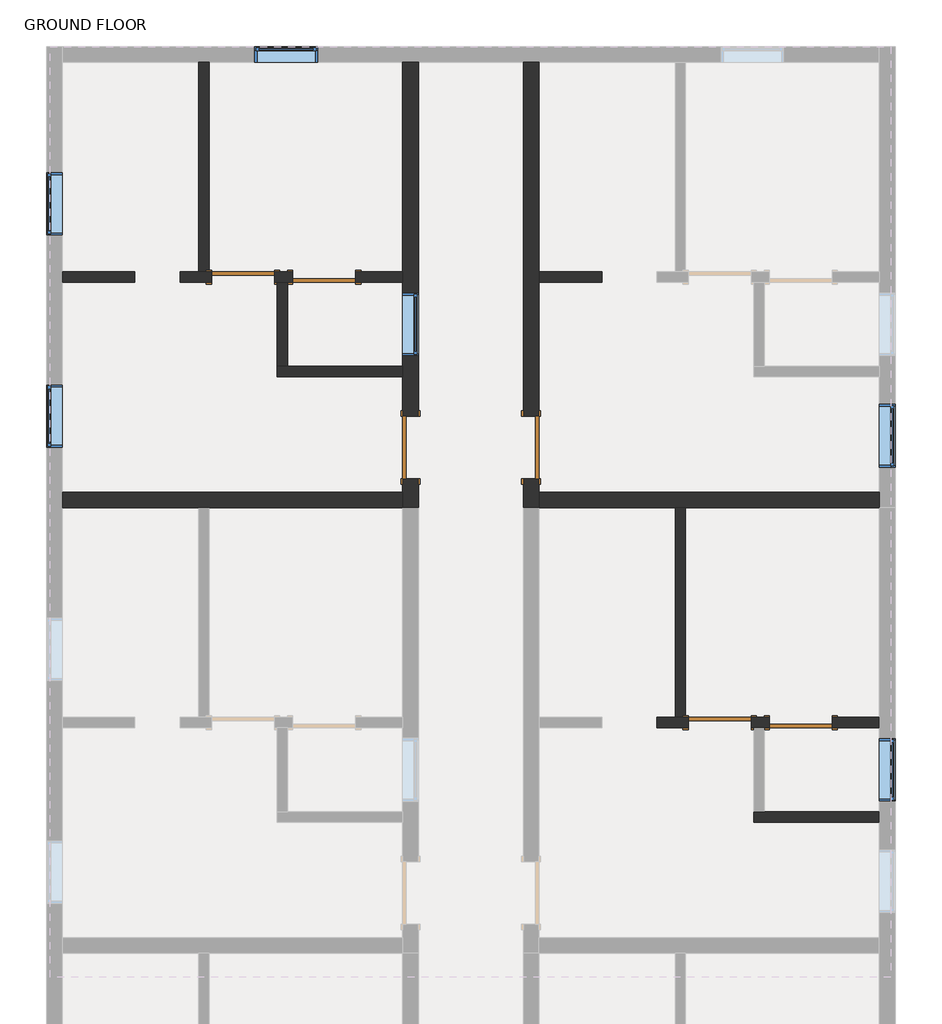
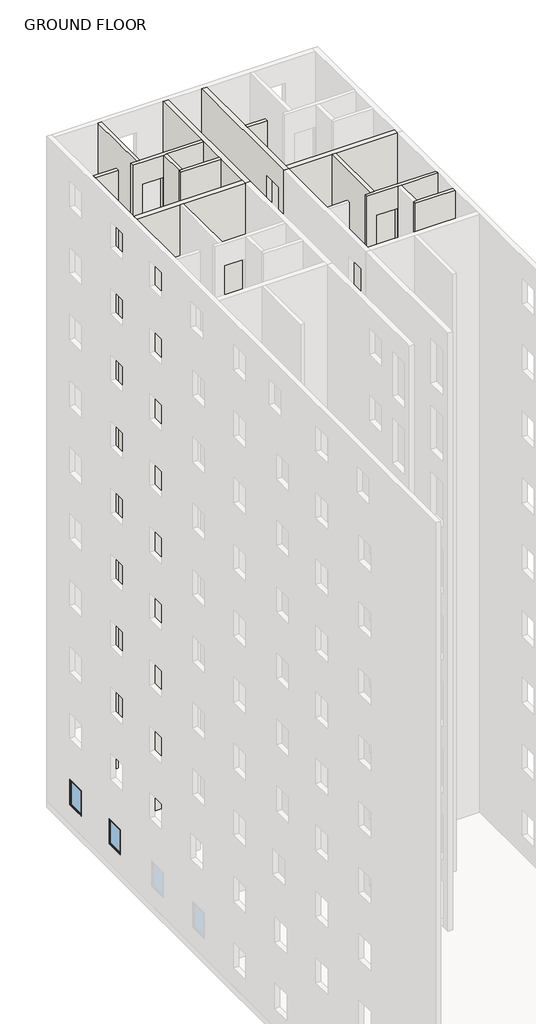
# One storey, part 6 of 7: 13 walls, 6 doors, 6 windows.
"""IFC4 building model written with IfcOpenShell, lengths in millimetres."""

from ifc_helpers import new_model, si_unit, origin, origin_with_axes, place, context, project, spatial, polyline, outline, extrude, faceted_brep, transform, mapped, element, save
from components import door_686f89d2, door_16372e1c, door_a90ba1ad, door_0ca8825f, window_c1f32544

model = new_model("IFC4")

# Units and contexts
model_context = context("Model", 3, world=origin())
ifc_project = project(units=[si_unit("LENGTHUNIT", "METRE", prefix="MILLI")], contexts=[model_context])

# Site, building, storey
site = spatial("IfcSite", under=ifc_project)
building = spatial("IfcBuilding", under=site)
storey = spatial("IfcBuildingStorey", under=building, Name="GROUND FLOOR", Elevation=0.0)

# Doors
placement = place(None, origin())
door_shape = door_686f89d2(model_context)
element("IfcDoor", 1, ObjectType="Single-Flush : 36\" x 84\"", at=placement, inside=storey, context=model_context, shape_type="MappedRepresentation", body=[
    mapped(door_shape, transform((-9863.5902461, 11952.2710592, 0.0), x_axis=(-1.0, 0.0, 0.0), y_axis=(0.0, -1.0, 0.0), z_axis=(0.0, 0.0, 1.0))),
])
element("IfcDoor", 2, ObjectType="Single-Flush : 36\" x 84\"", at=placement, inside=storey, context=model_context, shape_type="MappedRepresentation", body=[
    mapped(door_shape, transform((-2929.3902461, 5475.2710592, 0.0), x_axis=(-1.0, 0.0, 0.0), y_axis=(0.0, -1.0, 0.0), z_axis=(0.0, 0.0, 1.0))),
])
door_2_shape = door_16372e1c(model_context)
element("IfcDoor", 3, ObjectType="Single-Flush : 36\" x 84\"", at=placement, inside=storey, context=model_context, shape_type="MappedRepresentation", body=[
    mapped(door_2_shape, transform((-8682.4902461, 11952.2710592, 0.0), x_axis=(-1.0, 0.0, 0.0), y_axis=(0.0, -1.0, 0.0), z_axis=(0.0, 0.0, 1.0))),
])
element("IfcDoor", 4, ObjectType="Single-Flush : 36\" x 84\"", at=placement, inside=storey, context=model_context, shape_type="MappedRepresentation", body=[
    mapped(door_2_shape, transform((-1748.2902461, 5475.2710592, 0.0), x_axis=(-1.0, 0.0, 0.0), y_axis=(0.0, -1.0, 0.0), z_axis=(0.0, 0.0, 1.0))),
])
door_3_shape = door_a90ba1ad(model_context)
element("IfcDoor", 5, ObjectType="Single-Flush : 36\" x 84\"", at=placement, inside=storey, context=model_context, shape_type="MappedRepresentation", body=[
    mapped(door_3_shape, transform((-7425.1902461, 9475.7710592, 0.0), x_axis=(0.0, -1.0, 0.0), y_axis=(1.0, 0.0, 0.0), z_axis=(0.0, 0.0, 1.0))),
])
door_4_shape = door_0ca8825f(model_context)
element("IfcDoor", 6, ObjectType="Single-Flush : 36\" x 84\"", at=placement, inside=storey, context=model_context, shape_type="MappedRepresentation", body=[
    mapped(door_4_shape, transform((-5672.5902461, 9475.7710592, 0.0), x_axis=(0.0, -1.0, 0.0), y_axis=(1.0, 0.0, 0.0), z_axis=(0.0, 0.0, 1.0))),
])

# Walls
element("IfcWall", 7, ObjectType="Generic - 8\"", at=placement, inside=storey, context=model_context, shape_type="Brep", body=[
    faceted_brep([(-5558.2902461, 8599.4710592, 0.0), (-5558.2902461, 8828.0710592, 0.0), (-5558.2902461, 9018.5710592, 0.0), (-5558.2902461, 9018.5710592, 2133.6), (-5558.2902461, 9932.9710592, 2133.6), (-5558.2902461, 9932.9710592, 0.0), (-5558.2902461, 11876.0710592, 0.0), (-5558.2902461, 12028.4710592, 0.0), (-5558.2902461, 15076.4710592, 0.0), (-5558.2902461, 15076.4710592, 32004.0), (-5558.2902461, 12028.4710592, 32004.0), (-5558.2902461, 11876.0710592, 32004.0), (-5558.2902461, 8828.0710592, 32004.0), (-5558.2902461, 8599.4710592, 32004.0), (-5558.2902461, 9932.9710592, 3200.4), (-5558.2902461, 9018.5710592, 3200.4), (-5558.2902461, 9018.5710592, 5334.0), (-5558.2902461, 9932.9710592, 5334.0), (-5558.2902461, 9932.9710592, 6400.8), (-5558.2902461, 9018.5710592, 6400.8), (-5558.2902461, 9018.5710592, 8534.4), (-5558.2902461, 9932.9710592, 8534.4), (-5558.2902461, 9932.9710592, 9601.2), (-5558.2902461, 9018.5710592, 9601.2), (-5558.2902461, 9018.5710592, 11734.8), (-5558.2902461, 9932.9710592, 11734.8), (-5558.2902461, 9932.9710592, 12801.6), (-5558.2902461, 9018.5710592, 12801.6), (-5558.2902461, 9018.5710592, 14935.2), (-5558.2902461, 9932.9710592, 14935.2), (-5558.2902461, 9932.9710592, 16002.0), (-5558.2902461, 9018.5710592, 16002.0), (-5558.2902461, 9018.5710592, 18135.6), (-5558.2902461, 9932.9710592, 18135.6), (-5558.2902461, 9932.9710592, 19202.4), (-5558.2902461, 9018.5710592, 19202.4), (-5558.2902461, 9018.5710592, 21336.0), (-5558.2902461, 9932.9710592, 21336.0), (-5558.2902461, 9932.9710592, 22402.8), (-5558.2902461, 9018.5710592, 22402.8), (-5558.2902461, 9018.5710592, 24536.4), (-5558.2902461, 9932.9710592, 24536.4), (-5558.2902461, 9932.9710592, 25603.2), (-5558.2902461, 9018.5710592, 25603.2), (-5558.2902461, 9018.5710592, 27736.8), (-5558.2902461, 9932.9710592, 27736.8), (-5558.2902461, 9932.9710592, 28803.6), (-5558.2902461, 9018.5710592, 28803.6), (-5558.2902461, 9018.5710592, 30937.2), (-5558.2902461, 9932.9710592, 30937.2), (-5786.8902461, 9018.5710592, 2133.6), (-5786.8902461, 9018.5710592, 0.0), (-5786.8902461, 8599.4710592, 0.0), (-5786.8902461, 8599.4710592, 32004.0), (-5786.8902461, 15076.4710592, 32004.0), (-5786.8902461, 15076.4710592, 0.0), (-5786.8902461, 9932.9710592, 0.0), (-5786.8902461, 9932.9710592, 2133.6), (-5786.8902461, 9932.9710592, 3200.4), (-5786.8902461, 9932.9710592, 5334.0), (-5786.8902461, 9018.5710592, 5334.0), (-5786.8902461, 9018.5710592, 3200.4), (-5786.8902461, 9932.9710592, 6400.8), (-5786.8902461, 9932.9710592, 8534.4), (-5786.8902461, 9018.5710592, 8534.4), (-5786.8902461, 9018.5710592, 6400.8), (-5786.8902461, 9932.9710592, 9601.2), (-5786.8902461, 9932.9710592, 11734.8), (-5786.8902461, 9018.5710592, 11734.8), (-5786.8902461, 9018.5710592, 9601.2), (-5786.8902461, 9932.9710592, 12801.6), (-5786.8902461, 9932.9710592, 14935.2), (-5786.8902461, 9018.5710592, 14935.2), (-5786.8902461, 9018.5710592, 12801.6), (-5786.8902461, 9932.9710592, 16002.0), (-5786.8902461, 9932.9710592, 18135.6), (-5786.8902461, 9018.5710592, 18135.6), (-5786.8902461, 9018.5710592, 16002.0), (-5786.8902461, 9932.9710592, 19202.4), (-5786.8902461, 9932.9710592, 21336.0), (-5786.8902461, 9018.5710592, 21336.0), (-5786.8902461, 9018.5710592, 19202.4), (-5786.8902461, 9932.9710592, 22402.8), (-5786.8902461, 9932.9710592, 24536.4), (-5786.8902461, 9018.5710592, 24536.4), (-5786.8902461, 9018.5710592, 22402.8), (-5786.8902461, 9932.9710592, 25603.2), (-5786.8902461, 9932.9710592, 27736.8), (-5786.8902461, 9018.5710592, 27736.8), (-5786.8902461, 9018.5710592, 25603.2), (-5786.8902461, 9932.9710592, 28803.6), (-5786.8902461, 9932.9710592, 30937.2), (-5786.8902461, 9018.5710592, 30937.2), (-5786.8902461, 9018.5710592, 28803.6)], [[[0, 1, 2, 3, 4, 5, 6, 7, 8, 9, 10, 11, 12, 13], [14, 15, 16, 17], [18, 19, 20, 21], [22, 23, 24, 25], [26, 27, 28, 29], [30, 31, 32, 33], [34, 35, 36, 37], [38, 39, 40, 41], [42, 43, 44, 45], [46, 47, 48, 49]], [[50, 51, 52, 53, 54, 55, 56, 57], [58, 59, 60, 61], [62, 63, 64, 65], [66, 67, 68, 69], [70, 71, 72, 73], [74, 75, 76, 77], [78, 79, 80, 81], [82, 83, 84, 85], [86, 87, 88, 89], [90, 91, 92, 93]], [[56, 55, 8, 7, 6, 5]], [[52, 51, 2, 1, 0]], [[13, 12, 11, 10, 9, 54, 53]], [[0, 13, 53, 52]], [[9, 8, 55, 54]], [[3, 2, 51, 50]], [[4, 3, 50, 57]], [[5, 4, 57, 56]], [[15, 14, 58, 61]], [[16, 15, 61, 60]], [[17, 16, 60, 59]], [[14, 17, 59, 58]], [[19, 18, 62, 65]], [[20, 19, 65, 64]], [[21, 20, 64, 63]], [[18, 21, 63, 62]], [[23, 22, 66, 69]], [[24, 23, 69, 68]], [[25, 24, 68, 67]], [[22, 25, 67, 66]], [[27, 26, 70, 73]], [[28, 27, 73, 72]], [[29, 28, 72, 71]], [[26, 29, 71, 70]], [[31, 30, 74, 77]], [[32, 31, 77, 76]], [[33, 32, 76, 75]], [[30, 33, 75, 74]], [[35, 34, 78, 81]], [[36, 35, 81, 80]], [[37, 36, 80, 79]], [[34, 37, 79, 78]], [[39, 38, 82, 85]], [[40, 39, 85, 84]], [[41, 40, 84, 83]], [[38, 41, 83, 82]], [[43, 42, 86, 89]], [[44, 43, 89, 88]], [[45, 44, 88, 87]], [[42, 45, 87, 86]], [[47, 46, 90, 93]], [[48, 47, 93, 92]], [[49, 48, 92, 91]], [[46, 49, 91, 90]]]),
])
element("IfcWall", 8, ObjectType="INNER WALL 2", at=placement, inside=storey, context=model_context, shape_type="Brep", body=[
    faceted_brep([(-9406.3902461, 11876.0710592, 0.0), (-9368.2902461, 11876.0710592, 0.0), (-9215.8902461, 11876.0710592, 0.0), (-9139.6902461, 11876.0710592, 0.0), (-9139.6902461, 11876.0710592, 2133.6), (-8225.2902461, 11876.0710592, 2133.6), (-8225.2902461, 11876.0710592, 0.0), (-7539.4902461, 11876.0710592, 0.0), (-7539.4902461, 11876.0710592, 32004.0), (-9215.8902461, 11876.0710592, 32004.0), (-9368.2902461, 11876.0710592, 32004.0), (-10777.9902461, 11876.0710592, 32004.0), (-10777.9902461, 11876.0710592, 0.0), (-10320.7902461, 11876.0710592, 0.0), (-10320.7902461, 11876.0710592, 2133.6), (-9406.3902461, 11876.0710592, 2133.6), (-9406.3902461, 11876.0710592, 3200.4), (-10320.7902461, 11876.0710592, 3200.4), (-10320.7902461, 11876.0710592, 5334.0), (-9406.3902461, 11876.0710592, 5334.0), (-8225.2902461, 11876.0710592, 3200.4), (-9139.6902461, 11876.0710592, 3200.4), (-9139.6902461, 11876.0710592, 5334.0), (-8225.2902461, 11876.0710592, 5334.0), (-9406.3902461, 11876.0710592, 6400.8), (-10320.7902461, 11876.0710592, 6400.8), (-10320.7902461, 11876.0710592, 8534.4), (-9406.3902461, 11876.0710592, 8534.4), (-8225.2902461, 11876.0710592, 6400.8), (-9139.6902461, 11876.0710592, 6400.8), (-9139.6902461, 11876.0710592, 8534.4), (-8225.2902461, 11876.0710592, 8534.4), (-9406.3902461, 11876.0710592, 9601.2), (-10320.7902461, 11876.0710592, 9601.2), (-10320.7902461, 11876.0710592, 11734.8), (-9406.3902461, 11876.0710592, 11734.8), (-8225.2902461, 11876.0710592, 9601.2), (-9139.6902461, 11876.0710592, 9601.2), (-9139.6902461, 11876.0710592, 11734.8), (-8225.2902461, 11876.0710592, 11734.8), (-9406.3902461, 11876.0710592, 12801.6), (-10320.7902461, 11876.0710592, 12801.6), (-10320.7902461, 11876.0710592, 14935.2), (-9406.3902461, 11876.0710592, 14935.2), (-8225.2902461, 11876.0710592, 12801.6), (-9139.6902461, 11876.0710592, 12801.6), (-9139.6902461, 11876.0710592, 14935.2), (-8225.2902461, 11876.0710592, 14935.2), (-9406.3902461, 11876.0710592, 16002.0), (-10320.7902461, 11876.0710592, 16002.0), (-10320.7902461, 11876.0710592, 18135.6), (-9406.3902461, 11876.0710592, 18135.6), (-8225.2902461, 11876.0710592, 16002.0), (-9139.6902461, 11876.0710592, 16002.0), (-9139.6902461, 11876.0710592, 18135.6), (-8225.2902461, 11876.0710592, 18135.6), (-9406.3902461, 11876.0710592, 19202.4), (-10320.7902461, 11876.0710592, 19202.4), (-10320.7902461, 11876.0710592, 21336.0), (-9406.3902461, 11876.0710592, 21336.0), (-8225.2902461, 11876.0710592, 19202.4), (-9139.6902461, 11876.0710592, 19202.4), (-9139.6902461, 11876.0710592, 21336.0), (-8225.2902461, 11876.0710592, 21336.0), (-9406.3902461, 11876.0710592, 22402.8), (-10320.7902461, 11876.0710592, 22402.8), (-10320.7902461, 11876.0710592, 24536.4), (-9406.3902461, 11876.0710592, 24536.4), (-8225.2902461, 11876.0710592, 22402.8), (-9139.6902461, 11876.0710592, 22402.8), (-9139.6902461, 11876.0710592, 24536.4), (-8225.2902461, 11876.0710592, 24536.4), (-9406.3902461, 11876.0710592, 25603.2), (-10320.7902461, 11876.0710592, 25603.2), (-10320.7902461, 11876.0710592, 27736.8), (-9406.3902461, 11876.0710592, 27736.8), (-8225.2902461, 11876.0710592, 25603.2), (-9139.6902461, 11876.0710592, 25603.2), (-9139.6902461, 11876.0710592, 27736.8), (-8225.2902461, 11876.0710592, 27736.8), (-9406.3902461, 11876.0710592, 28803.6), (-10320.7902461, 11876.0710592, 28803.6), (-10320.7902461, 11876.0710592, 30937.2), (-9406.3902461, 11876.0710592, 30937.2), (-8225.2902461, 11876.0710592, 28803.6), (-9139.6902461, 11876.0710592, 28803.6), (-9139.6902461, 11876.0710592, 30937.2), (-8225.2902461, 11876.0710592, 30937.2), (-9139.6902461, 12028.4710592, 2133.6), (-9139.6902461, 12028.4710592, 0.0), (-9406.3902461, 12028.4710592, 0.0), (-9406.3902461, 12028.4710592, 2133.6), (-10320.7902461, 12028.4710592, 2133.6), (-10320.7902461, 12028.4710592, 0.0), (-10358.8902461, 12028.4710592, 0.0), (-10511.2902461, 12028.4710592, 0.0), (-10777.9902461, 12028.4710592, 0.0), (-10777.9902461, 12028.4710592, 32004.0), (-10511.2902461, 12028.4710592, 32004.0), (-10358.8902461, 12028.4710592, 32004.0), (-7539.4902461, 12028.4710592, 32004.0), (-7539.4902461, 12028.4710592, 0.0), (-8225.2902461, 12028.4710592, 0.0), (-8225.2902461, 12028.4710592, 2133.6), (-9406.3902461, 12028.4710592, 3200.4), (-9406.3902461, 12028.4710592, 5334.0), (-10320.7902461, 12028.4710592, 5334.0), (-10320.7902461, 12028.4710592, 3200.4), (-8225.2902461, 12028.4710592, 3200.4), (-8225.2902461, 12028.4710592, 5334.0), (-9139.6902461, 12028.4710592, 5334.0), (-9139.6902461, 12028.4710592, 3200.4), (-9406.3902461, 12028.4710592, 6400.8), (-9406.3902461, 12028.4710592, 8534.4), (-10320.7902461, 12028.4710592, 8534.4), (-10320.7902461, 12028.4710592, 6400.8), (-8225.2902461, 12028.4710592, 6400.8), (-8225.2902461, 12028.4710592, 8534.4), (-9139.6902461, 12028.4710592, 8534.4), (-9139.6902461, 12028.4710592, 6400.8), (-9406.3902461, 12028.4710592, 9601.2), (-9406.3902461, 12028.4710592, 11734.8), (-10320.7902461, 12028.4710592, 11734.8), (-10320.7902461, 12028.4710592, 9601.2), (-8225.2902461, 12028.4710592, 9601.2), (-8225.2902461, 12028.4710592, 11734.8), (-9139.6902461, 12028.4710592, 11734.8), (-9139.6902461, 12028.4710592, 9601.2), (-9406.3902461, 12028.4710592, 12801.6), (-9406.3902461, 12028.4710592, 14935.2), (-10320.7902461, 12028.4710592, 14935.2), (-10320.7902461, 12028.4710592, 12801.6), (-8225.2902461, 12028.4710592, 12801.6), (-8225.2902461, 12028.4710592, 14935.2), (-9139.6902461, 12028.4710592, 14935.2), (-9139.6902461, 12028.4710592, 12801.6), (-9406.3902461, 12028.4710592, 16002.0), (-9406.3902461, 12028.4710592, 18135.6), (-10320.7902461, 12028.4710592, 18135.6), (-10320.7902461, 12028.4710592, 16002.0), (-8225.2902461, 12028.4710592, 16002.0), (-8225.2902461, 12028.4710592, 18135.6), (-9139.6902461, 12028.4710592, 18135.6), (-9139.6902461, 12028.4710592, 16002.0), (-9406.3902461, 12028.4710592, 19202.4), (-9406.3902461, 12028.4710592, 21336.0), (-10320.7902461, 12028.4710592, 21336.0), (-10320.7902461, 12028.4710592, 19202.4), (-8225.2902461, 12028.4710592, 19202.4), (-8225.2902461, 12028.4710592, 21336.0), (-9139.6902461, 12028.4710592, 21336.0), (-9139.6902461, 12028.4710592, 19202.4), (-9406.3902461, 12028.4710592, 22402.8), (-9406.3902461, 12028.4710592, 24536.4), (-10320.7902461, 12028.4710592, 24536.4), (-10320.7902461, 12028.4710592, 22402.8), (-8225.2902461, 12028.4710592, 22402.8), (-8225.2902461, 12028.4710592, 24536.4), (-9139.6902461, 12028.4710592, 24536.4), (-9139.6902461, 12028.4710592, 22402.8), (-9406.3902461, 12028.4710592, 25603.2), (-9406.3902461, 12028.4710592, 27736.8), (-10320.7902461, 12028.4710592, 27736.8), (-10320.7902461, 12028.4710592, 25603.2), (-8225.2902461, 12028.4710592, 25603.2), (-8225.2902461, 12028.4710592, 27736.8), (-9139.6902461, 12028.4710592, 27736.8), (-9139.6902461, 12028.4710592, 25603.2), (-9406.3902461, 12028.4710592, 28803.6), (-9406.3902461, 12028.4710592, 30937.2), (-10320.7902461, 12028.4710592, 30937.2), (-10320.7902461, 12028.4710592, 28803.6), (-8225.2902461, 12028.4710592, 28803.6), (-8225.2902461, 12028.4710592, 30937.2), (-9139.6902461, 12028.4710592, 30937.2), (-9139.6902461, 12028.4710592, 28803.6)], [[[0, 1, 2, 3, 4, 5, 6, 7, 8, 9, 10, 11, 12, 13, 14, 15], [16, 17, 18, 19], [20, 21, 22, 23], [24, 25, 26, 27], [28, 29, 30, 31], [32, 33, 34, 35], [36, 37, 38, 39], [40, 41, 42, 43], [44, 45, 46, 47], [48, 49, 50, 51], [52, 53, 54, 55], [56, 57, 58, 59], [60, 61, 62, 63], [64, 65, 66, 67], [68, 69, 70, 71], [72, 73, 74, 75], [76, 77, 78, 79], [80, 81, 82, 83], [84, 85, 86, 87]], [[88, 89, 90, 91, 92, 93, 94, 95, 96, 97, 98, 99, 100, 101, 102, 103], [104, 105, 106, 107], [108, 109, 110, 111], [112, 113, 114, 115], [116, 117, 118, 119], [120, 121, 122, 123], [124, 125, 126, 127], [128, 129, 130, 131], [132, 133, 134, 135], [136, 137, 138, 139], [140, 141, 142, 143], [144, 145, 146, 147], [148, 149, 150, 151], [152, 153, 154, 155], [156, 157, 158, 159], [160, 161, 162, 163], [164, 165, 166, 167], [168, 169, 170, 171], [172, 173, 174, 175]], [[96, 95, 94, 93, 13, 12]], [[102, 101, 7, 6]], [[90, 89, 3, 2, 1, 0]], [[11, 10, 9, 8, 100, 99, 98, 97]], [[12, 11, 97, 96]], [[8, 7, 101, 100]], [[14, 13, 93, 92]], [[15, 14, 92, 91]], [[0, 15, 91, 90]], [[4, 3, 89, 88]], [[5, 4, 88, 103]], [[6, 5, 103, 102]], [[17, 16, 104, 107]], [[18, 17, 107, 106]], [[19, 18, 106, 105]], [[16, 19, 105, 104]], [[21, 20, 108, 111]], [[22, 21, 111, 110]], [[23, 22, 110, 109]], [[20, 23, 109, 108]], [[25, 24, 112, 115]], [[26, 25, 115, 114]], [[27, 26, 114, 113]], [[24, 27, 113, 112]], [[29, 28, 116, 119]], [[30, 29, 119, 118]], [[31, 30, 118, 117]], [[28, 31, 117, 116]], [[33, 32, 120, 123]], [[34, 33, 123, 122]], [[35, 34, 122, 121]], [[32, 35, 121, 120]], [[37, 36, 124, 127]], [[38, 37, 127, 126]], [[39, 38, 126, 125]], [[36, 39, 125, 124]], [[41, 40, 128, 131]], [[42, 41, 131, 130]], [[43, 42, 130, 129]], [[40, 43, 129, 128]], [[45, 44, 132, 135]], [[46, 45, 135, 134]], [[47, 46, 134, 133]], [[44, 47, 133, 132]], [[49, 48, 136, 139]], [[50, 49, 139, 138]], [[51, 50, 138, 137]], [[48, 51, 137, 136]], [[53, 52, 140, 143]], [[54, 53, 143, 142]], [[55, 54, 142, 141]], [[52, 55, 141, 140]], [[57, 56, 144, 147]], [[58, 57, 147, 146]], [[59, 58, 146, 145]], [[56, 59, 145, 144]], [[61, 60, 148, 151]], [[62, 61, 151, 150]], [[63, 62, 150, 149]], [[60, 63, 149, 148]], [[65, 64, 152, 155]], [[66, 65, 155, 154]], [[67, 66, 154, 153]], [[64, 67, 153, 152]], [[69, 68, 156, 159]], [[70, 69, 159, 158]], [[71, 70, 158, 157]], [[68, 71, 157, 156]], [[73, 72, 160, 163]], [[74, 73, 163, 162]], [[75, 74, 162, 161]], [[72, 75, 161, 160]], [[77, 76, 164, 167]], [[78, 77, 167, 166]], [[79, 78, 166, 165]], [[76, 79, 165, 164]], [[81, 80, 168, 171]], [[82, 81, 171, 170]], [[83, 82, 170, 169]], [[80, 83, 169, 168]], [[85, 84, 172, 175]], [[86, 85, 175, 174]], [[87, 86, 174, 173]], [[84, 87, 173, 172]]]),
])
element("IfcWall", 9, ObjectType="INNER WALL 2", at=placement, inside=storey, context=model_context, shape_type="SweptSolid", body=[
    extrude(outline(polyline([(-10358.8902461, 15076.4710592), (-10358.8902461, 12028.4710592), (-10511.2902461, 12028.4710592), (-10511.2902461, 15076.4710592), (-10358.8902461, 15076.4710592)])), origin_with_axes(), (0.0, 0.0, 1.0), 32004.0),
])
element("IfcWall", 10, ObjectType="INNER WALL 2", at=placement, inside=storey, context=model_context, shape_type="Brep", body=[
    faceted_brep([(-7539.4902461, 10656.8710592, 0.0), (-9215.8902461, 10656.8710592, 0.0), (-9368.2902461, 10656.8710592, 0.0), (-9368.2902461, 10656.8710592, 32004.0), (-9215.8902461, 10656.8710592, 32004.0), (-7539.4902461, 10656.8710592, 32004.0), (-7539.4902461, 10504.4710592, 0.0), (-7539.4902461, 10504.4710592, 32004.0), (-9368.2902461, 10504.4710592, 32004.0), (-9368.2902461, 10504.4710592, 0.0)], [[[0, 1, 2, 3, 4, 5]], [[6, 7, 8, 9]], [[2, 1, 0, 6, 9]], [[5, 4, 3, 8, 7]], [[0, 5, 7, 6]], [[3, 2, 9, 8]]]),
])
element("IfcWall", 11, ObjectType="INNER WALL 2", at=placement, inside=storey, context=model_context, shape_type="SweptSolid", body=[
    extrude(outline(polyline([(-9215.8902461, 11876.0710592), (-9215.8902461, 10656.8710592), (-9368.2902461, 10656.8710592), (-9368.2902461, 11876.0710592), (-9215.8902461, 11876.0710592)])), origin_with_axes(), (0.0, 0.0, 1.0), 32004.0),
])
element("IfcWall", 12, ObjectType="INNER WALL 2", at=placement, inside=storey, context=model_context, shape_type="Brep", body=[
    faceted_brep([(-2472.1902461, 5399.0710592, 0.0), (-2434.0902461, 5399.0710592, 0.0), (-2281.6902461, 5399.0710592, 0.0), (-2205.4902461, 5399.0710592, 0.0), (-2205.4902461, 5399.0710592, 2133.6), (-1291.0902461, 5399.0710592, 2133.6), (-1291.0902461, 5399.0710592, 0.0), (-605.2902461, 5399.0710592, 0.0), (-605.2902461, 5399.0710592, 32004.0), (-2281.6902461, 5399.0710592, 32004.0), (-2434.0902461, 5399.0710592, 32004.0), (-3843.7902461, 5399.0710592, 32004.0), (-3843.7902461, 5399.0710592, 0.0), (-3386.5902461, 5399.0710592, 0.0), (-3386.5902461, 5399.0710592, 2133.6), (-2472.1902461, 5399.0710592, 2133.6), (-1291.0902461, 5399.0710592, 3200.4), (-2205.4902461, 5399.0710592, 3200.4), (-2205.4902461, 5399.0710592, 5334.0), (-1291.0902461, 5399.0710592, 5334.0), (-2472.1902461, 5399.0710592, 3200.4), (-3386.5902461, 5399.0710592, 3200.4), (-3386.5902461, 5399.0710592, 5334.0), (-2472.1902461, 5399.0710592, 5334.0), (-2472.1902461, 5399.0710592, 6400.8), (-3386.5902461, 5399.0710592, 6400.8), (-3386.5902461, 5399.0710592, 8534.4), (-2472.1902461, 5399.0710592, 8534.4), (-1291.0902461, 5399.0710592, 6400.8), (-2205.4902461, 5399.0710592, 6400.8), (-2205.4902461, 5399.0710592, 8534.4), (-1291.0902461, 5399.0710592, 8534.4), (-2472.1902461, 5399.0710592, 9601.2), (-3386.5902461, 5399.0710592, 9601.2), (-3386.5902461, 5399.0710592, 11734.8), (-2472.1902461, 5399.0710592, 11734.8), (-1291.0902461, 5399.0710592, 9601.2), (-2205.4902461, 5399.0710592, 9601.2), (-2205.4902461, 5399.0710592, 11734.8), (-1291.0902461, 5399.0710592, 11734.8), (-1291.0902461, 5399.0710592, 12801.6), (-2205.4902461, 5399.0710592, 12801.6), (-2205.4902461, 5399.0710592, 14935.2), (-1291.0902461, 5399.0710592, 14935.2), (-2472.1902461, 5399.0710592, 12801.6), (-3386.5902461, 5399.0710592, 12801.6), (-3386.5902461, 5399.0710592, 14935.2), (-2472.1902461, 5399.0710592, 14935.2), (-1291.0902461, 5399.0710592, 16002.0), (-2205.4902461, 5399.0710592, 16002.0), (-2205.4902461, 5399.0710592, 18135.6), (-1291.0902461, 5399.0710592, 18135.6), (-2472.1902461, 5399.0710592, 16002.0), (-3386.5902461, 5399.0710592, 16002.0), (-3386.5902461, 5399.0710592, 18135.6), (-2472.1902461, 5399.0710592, 18135.6), (-1291.0902461, 5399.0710592, 19202.4), (-2205.4902461, 5399.0710592, 19202.4), (-2205.4902461, 5399.0710592, 21336.0), (-1291.0902461, 5399.0710592, 21336.0), (-2472.1902461, 5399.0710592, 19202.4), (-3386.5902461, 5399.0710592, 19202.4), (-3386.5902461, 5399.0710592, 21336.0), (-2472.1902461, 5399.0710592, 21336.0), (-1291.0902461, 5399.0710592, 22402.8), (-2205.4902461, 5399.0710592, 22402.8), (-2205.4902461, 5399.0710592, 24536.4), (-1291.0902461, 5399.0710592, 24536.4), (-2472.1902461, 5399.0710592, 22402.8), (-3386.5902461, 5399.0710592, 22402.8), (-3386.5902461, 5399.0710592, 24536.4), (-2472.1902461, 5399.0710592, 24536.4), (-2472.1902461, 5399.0710592, 25603.2), (-3386.5902461, 5399.0710592, 25603.2), (-3386.5902461, 5399.0710592, 27736.8), (-2472.1902461, 5399.0710592, 27736.8), (-1291.0902461, 5399.0710592, 25603.2), (-2205.4902461, 5399.0710592, 25603.2), (-2205.4902461, 5399.0710592, 27736.8), (-1291.0902461, 5399.0710592, 27736.8), (-2472.1902461, 5399.0710592, 28803.6), (-3386.5902461, 5399.0710592, 28803.6), (-3386.5902461, 5399.0710592, 30937.2), (-2472.1902461, 5399.0710592, 30937.2), (-1291.0902461, 5399.0710592, 28803.6), (-2205.4902461, 5399.0710592, 28803.6), (-2205.4902461, 5399.0710592, 30937.2), (-1291.0902461, 5399.0710592, 30937.2), (-2205.4902461, 5551.4710592, 2133.6), (-2205.4902461, 5551.4710592, 0.0), (-2472.1902461, 5551.4710592, 0.0), (-2472.1902461, 5551.4710592, 2133.6), (-3386.5902461, 5551.4710592, 2133.6), (-3386.5902461, 5551.4710592, 0.0), (-3424.6902461, 5551.4710592, 0.0), (-3577.0902461, 5551.4710592, 0.0), (-3843.7902461, 5551.4710592, 0.0), (-3843.7902461, 5551.4710592, 32004.0), (-3577.0902461, 5551.4710592, 32004.0), (-3424.6902461, 5551.4710592, 32004.0), (-605.2902461, 5551.4710592, 32004.0), (-605.2902461, 5551.4710592, 0.0), (-1291.0902461, 5551.4710592, 0.0), (-1291.0902461, 5551.4710592, 2133.6), (-1291.0902461, 5551.4710592, 3200.4), (-1291.0902461, 5551.4710592, 5334.0), (-2205.4902461, 5551.4710592, 5334.0), (-2205.4902461, 5551.4710592, 3200.4), (-2472.1902461, 5551.4710592, 3200.4), (-2472.1902461, 5551.4710592, 5334.0), (-3386.5902461, 5551.4710592, 5334.0), (-3386.5902461, 5551.4710592, 3200.4), (-2472.1902461, 5551.4710592, 6400.8), (-2472.1902461, 5551.4710592, 8534.4), (-3386.5902461, 5551.4710592, 8534.4), (-3386.5902461, 5551.4710592, 6400.8), (-1291.0902461, 5551.4710592, 6400.8), (-1291.0902461, 5551.4710592, 8534.4), (-2205.4902461, 5551.4710592, 8534.4), (-2205.4902461, 5551.4710592, 6400.8), (-2472.1902461, 5551.4710592, 9601.2), (-2472.1902461, 5551.4710592, 11734.8), (-3386.5902461, 5551.4710592, 11734.8), (-3386.5902461, 5551.4710592, 9601.2), (-1291.0902461, 5551.4710592, 9601.2), (-1291.0902461, 5551.4710592, 11734.8), (-2205.4902461, 5551.4710592, 11734.8), (-2205.4902461, 5551.4710592, 9601.2), (-1291.0902461, 5551.4710592, 12801.6), (-1291.0902461, 5551.4710592, 14935.2), (-2205.4902461, 5551.4710592, 14935.2), (-2205.4902461, 5551.4710592, 12801.6), (-2472.1902461, 5551.4710592, 12801.6), (-2472.1902461, 5551.4710592, 14935.2), (-3386.5902461, 5551.4710592, 14935.2), (-3386.5902461, 5551.4710592, 12801.6), (-1291.0902461, 5551.4710592, 16002.0), (-1291.0902461, 5551.4710592, 18135.6), (-2205.4902461, 5551.4710592, 18135.6), (-2205.4902461, 5551.4710592, 16002.0), (-2472.1902461, 5551.4710592, 16002.0), (-2472.1902461, 5551.4710592, 18135.6), (-3386.5902461, 5551.4710592, 18135.6), (-3386.5902461, 5551.4710592, 16002.0), (-1291.0902461, 5551.4710592, 19202.4), (-1291.0902461, 5551.4710592, 21336.0), (-2205.4902461, 5551.4710592, 21336.0), (-2205.4902461, 5551.4710592, 19202.4), (-2472.1902461, 5551.4710592, 19202.4), (-2472.1902461, 5551.4710592, 21336.0), (-3386.5902461, 5551.4710592, 21336.0), (-3386.5902461, 5551.4710592, 19202.4), (-1291.0902461, 5551.4710592, 22402.8), (-1291.0902461, 5551.4710592, 24536.4), (-2205.4902461, 5551.4710592, 24536.4), (-2205.4902461, 5551.4710592, 22402.8), (-2472.1902461, 5551.4710592, 22402.8), (-2472.1902461, 5551.4710592, 24536.4), (-3386.5902461, 5551.4710592, 24536.4), (-3386.5902461, 5551.4710592, 22402.8), (-2472.1902461, 5551.4710592, 25603.2), (-2472.1902461, 5551.4710592, 27736.8), (-3386.5902461, 5551.4710592, 27736.8), (-3386.5902461, 5551.4710592, 25603.2), (-1291.0902461, 5551.4710592, 25603.2), (-1291.0902461, 5551.4710592, 27736.8), (-2205.4902461, 5551.4710592, 27736.8), (-2205.4902461, 5551.4710592, 25603.2), (-2472.1902461, 5551.4710592, 28803.6), (-2472.1902461, 5551.4710592, 30937.2), (-3386.5902461, 5551.4710592, 30937.2), (-3386.5902461, 5551.4710592, 28803.6), (-1291.0902461, 5551.4710592, 28803.6), (-1291.0902461, 5551.4710592, 30937.2), (-2205.4902461, 5551.4710592, 30937.2), (-2205.4902461, 5551.4710592, 28803.6)], [[[0, 1, 2, 3, 4, 5, 6, 7, 8, 9, 10, 11, 12, 13, 14, 15], [16, 17, 18, 19], [20, 21, 22, 23], [24, 25, 26, 27], [28, 29, 30, 31], [32, 33, 34, 35], [36, 37, 38, 39], [40, 41, 42, 43], [44, 45, 46, 47], [48, 49, 50, 51], [52, 53, 54, 55], [56, 57, 58, 59], [60, 61, 62, 63], [64, 65, 66, 67], [68, 69, 70, 71], [72, 73, 74, 75], [76, 77, 78, 79], [80, 81, 82, 83], [84, 85, 86, 87]], [[88, 89, 90, 91, 92, 93, 94, 95, 96, 97, 98, 99, 100, 101, 102, 103], [104, 105, 106, 107], [108, 109, 110, 111], [112, 113, 114, 115], [116, 117, 118, 119], [120, 121, 122, 123], [124, 125, 126, 127], [128, 129, 130, 131], [132, 133, 134, 135], [136, 137, 138, 139], [140, 141, 142, 143], [144, 145, 146, 147], [148, 149, 150, 151], [152, 153, 154, 155], [156, 157, 158, 159], [160, 161, 162, 163], [164, 165, 166, 167], [168, 169, 170, 171], [172, 173, 174, 175]], [[96, 95, 94, 93, 13, 12]], [[102, 101, 7, 6]], [[90, 89, 3, 2, 1, 0]], [[11, 10, 9, 8, 100, 99, 98, 97]], [[12, 11, 97, 96]], [[8, 7, 101, 100]], [[14, 13, 93, 92]], [[15, 14, 92, 91]], [[0, 15, 91, 90]], [[4, 3, 89, 88]], [[5, 4, 88, 103]], [[6, 5, 103, 102]], [[17, 16, 104, 107]], [[18, 17, 107, 106]], [[19, 18, 106, 105]], [[16, 19, 105, 104]], [[21, 20, 108, 111]], [[22, 21, 111, 110]], [[23, 22, 110, 109]], [[20, 23, 109, 108]], [[25, 24, 112, 115]], [[26, 25, 115, 114]], [[27, 26, 114, 113]], [[24, 27, 113, 112]], [[29, 28, 116, 119]], [[30, 29, 119, 118]], [[31, 30, 118, 117]], [[28, 31, 117, 116]], [[33, 32, 120, 123]], [[34, 33, 123, 122]], [[35, 34, 122, 121]], [[32, 35, 121, 120]], [[37, 36, 124, 127]], [[38, 37, 127, 126]], [[39, 38, 126, 125]], [[36, 39, 125, 124]], [[41, 40, 128, 131]], [[42, 41, 131, 130]], [[43, 42, 130, 129]], [[40, 43, 129, 128]], [[45, 44, 132, 135]], [[46, 45, 135, 134]], [[47, 46, 134, 133]], [[44, 47, 133, 132]], [[49, 48, 136, 139]], [[50, 49, 139, 138]], [[51, 50, 138, 137]], [[48, 51, 137, 136]], [[53, 52, 140, 143]], [[54, 53, 143, 142]], [[55, 54, 142, 141]], [[52, 55, 141, 140]], [[57, 56, 144, 147]], [[58, 57, 147, 146]], [[59, 58, 146, 145]], [[56, 59, 145, 144]], [[61, 60, 148, 151]], [[62, 61, 151, 150]], [[63, 62, 150, 149]], [[60, 63, 149, 148]], [[65, 64, 152, 155]], [[66, 65, 155, 154]], [[67, 66, 154, 153]], [[64, 67, 153, 152]], [[69, 68, 156, 159]], [[70, 69, 159, 158]], [[71, 70, 158, 157]], [[68, 71, 157, 156]], [[73, 72, 160, 163]], [[74, 73, 163, 162]], [[75, 74, 162, 161]], [[72, 75, 161, 160]], [[77, 76, 164, 167]], [[78, 77, 167, 166]], [[79, 78, 166, 165]], [[76, 79, 165, 164]], [[81, 80, 168, 171]], [[82, 81, 171, 170]], [[83, 82, 170, 169]], [[80, 83, 169, 168]], [[85, 84, 172, 175]], [[86, 85, 175, 174]], [[87, 86, 174, 173]], [[84, 87, 173, 172]]]),
])
element("IfcWall", 13, ObjectType="INNER WALL 2", at=placement, inside=storey, context=model_context, shape_type="SweptSolid", body=[
    extrude(outline(polyline([(-3424.6902461, 8599.4710592), (-3424.6902461, 5551.4710592), (-3577.0902461, 5551.4710592), (-3577.0902461, 8599.4710592), (-3424.6902461, 8599.4710592)])), origin_with_axes(), (0.0, 0.0, 1.0), 32004.0),
])
element("IfcWall", 14, ObjectType="INNER WALL 2", at=placement, inside=storey, context=model_context, shape_type="Brep", body=[
    faceted_brep([(-605.2902461, 4179.8710592, 0.0), (-2281.6902461, 4179.8710592, 0.0), (-2434.0902461, 4179.8710592, 0.0), (-2434.0902461, 4179.8710592, 32004.0), (-2281.6902461, 4179.8710592, 32004.0), (-605.2902461, 4179.8710592, 32004.0), (-605.2902461, 4027.4710592, 0.0), (-605.2902461, 4027.4710592, 32004.0), (-2434.0902461, 4027.4710592, 32004.0), (-2434.0902461, 4027.4710592, 0.0)], [[[0, 1, 2, 3, 4, 5]], [[6, 7, 8, 9]], [[2, 1, 0, 6, 9]], [[5, 4, 3, 8, 7]], [[3, 2, 9, 8]], [[0, 5, 7, 6]]]),
])
element("IfcWall", 15, ObjectType="INNER WALL 2", at=placement, inside=storey, context=model_context, shape_type="SweptSolid", body=[
    extrude(outline(polyline([(-11438.3902461, 11876.0710592), (-12492.4902461, 11876.0710592), (-12492.4902461, 12028.4710592), (-11438.3902461, 12028.4710592), (-11438.3902461, 11876.0710592)])), origin_with_axes(), (0.0, 0.0, 1.0), 32004.0),
])
element("IfcWall", 16, ObjectType="INNER WALL 2", at=placement, inside=storey, context=model_context, shape_type="SweptSolid", body=[
    extrude(outline(polyline([(-4643.8902461, 11876.0710592), (-5558.2902461, 11876.0710592), (-5558.2902461, 12028.4710592), (-4643.8902461, 12028.4710592), (-4643.8902461, 11876.0710592)])), origin_with_axes(), (0.0, 0.0, 1.0), 32004.0),
])
element("IfcWall", 17, ObjectType="OUTER WALL", at=placement, inside=storey, context=model_context, shape_type="Brep", body=[
    faceted_brep([(-7310.8902461, 8599.4710592, 0.0), (-7310.8902461, 9018.5710592, 0.0), (-7310.8902461, 9018.5710592, 2133.6), (-7310.8902461, 9932.9710592, 2133.6), (-7310.8902461, 9932.9710592, 0.0), (-7310.8902461, 15076.4710592, 0.0), (-7310.8902461, 15076.4710592, 32004.0), (-7310.8902461, 8599.4710592, 32004.0), (-7310.8902461, 10809.2710592, 2133.6), (-7310.8902461, 11723.6710592, 2133.6), (-7310.8902461, 11723.6710592, 914.4), (-7310.8902461, 10809.2710592, 914.4), (-7310.8902461, 9932.9710592, 3200.4), (-7310.8902461, 9018.5710592, 3200.4), (-7310.8902461, 9018.5710592, 5334.0), (-7310.8902461, 9932.9710592, 5334.0), (-7310.8902461, 10809.2710592, 5334.0), (-7310.8902461, 11723.6710592, 5334.0), (-7310.8902461, 11723.6710592, 4114.8), (-7310.8902461, 10809.2710592, 4114.8), (-7310.8902461, 9932.9710592, 6400.8), (-7310.8902461, 9018.5710592, 6400.8), (-7310.8902461, 9018.5710592, 8534.4), (-7310.8902461, 9932.9710592, 8534.4), (-7310.8902461, 10809.2710592, 8534.4), (-7310.8902461, 11723.6710592, 8534.4), (-7310.8902461, 11723.6710592, 7315.2), (-7310.8902461, 10809.2710592, 7315.2), (-7310.8902461, 9932.9710592, 9601.2), (-7310.8902461, 9018.5710592, 9601.2), (-7310.8902461, 9018.5710592, 11734.8), (-7310.8902461, 9932.9710592, 11734.8), (-7310.8902461, 10809.2710592, 11734.8), (-7310.8902461, 11723.6710592, 11734.8), (-7310.8902461, 11723.6710592, 10515.6), (-7310.8902461, 10809.2710592, 10515.6), (-7310.8902461, 9932.9710592, 12801.6), (-7310.8902461, 9018.5710592, 12801.6), (-7310.8902461, 9018.5710592, 14935.2), (-7310.8902461, 9932.9710592, 14935.2), (-7310.8902461, 10809.2710592, 14935.2), (-7310.8902461, 11723.6710592, 14935.2), (-7310.8902461, 11723.6710592, 13716.0), (-7310.8902461, 10809.2710592, 13716.0), (-7310.8902461, 9932.9710592, 16002.0), (-7310.8902461, 9018.5710592, 16002.0), (-7310.8902461, 9018.5710592, 18135.6), (-7310.8902461, 9932.9710592, 18135.6), (-7310.8902461, 10809.2710592, 18135.6), (-7310.8902461, 11723.6710592, 18135.6), (-7310.8902461, 11723.6710592, 16916.4), (-7310.8902461, 10809.2710592, 16916.4), (-7310.8902461, 9932.9710592, 19202.4), (-7310.8902461, 9018.5710592, 19202.4), (-7310.8902461, 9018.5710592, 21336.0), (-7310.8902461, 9932.9710592, 21336.0), (-7310.8902461, 10809.2710592, 21336.0), (-7310.8902461, 11723.6710592, 21336.0), (-7310.8902461, 11723.6710592, 20116.8), (-7310.8902461, 10809.2710592, 20116.8), (-7310.8902461, 9932.9710592, 22402.8), (-7310.8902461, 9018.5710592, 22402.8), (-7310.8902461, 9018.5710592, 24536.4), (-7310.8902461, 9932.9710592, 24536.4), (-7310.8902461, 10809.2710592, 24536.4), (-7310.8902461, 11723.6710592, 24536.4), (-7310.8902461, 11723.6710592, 23317.2), (-7310.8902461, 10809.2710592, 23317.2), (-7310.8902461, 9932.9710592, 25603.2), (-7310.8902461, 9018.5710592, 25603.2), (-7310.8902461, 9018.5710592, 27736.8), (-7310.8902461, 9932.9710592, 27736.8), (-7310.8902461, 10809.2710592, 27736.8), (-7310.8902461, 11723.6710592, 27736.8), (-7310.8902461, 11723.6710592, 26517.6), (-7310.8902461, 10809.2710592, 26517.6), (-7310.8902461, 9932.9710592, 28803.6), (-7310.8902461, 9018.5710592, 28803.6), (-7310.8902461, 9018.5710592, 30937.2), (-7310.8902461, 9932.9710592, 30937.2), (-7310.8902461, 10809.2710592, 30937.2), (-7310.8902461, 11723.6710592, 30937.2), (-7310.8902461, 11723.6710592, 29718.0), (-7310.8902461, 10809.2710592, 29718.0), (-7539.4902461, 9018.5710592, 2133.6), (-7539.4902461, 9018.5710592, 0.0), (-7539.4902461, 8828.0710592, 0.0), (-7539.4902461, 8599.4710592, 0.0), (-7539.4902461, 8599.4710592, 32004.0), (-7539.4902461, 8828.0710592, 32004.0), (-7539.4902461, 10504.4710592, 32004.0), (-7539.4902461, 10656.8710592, 32004.0), (-7539.4902461, 11876.0710592, 32004.0), (-7539.4902461, 12028.4710592, 32004.0), (-7539.4902461, 15076.4710592, 32004.0), (-7539.4902461, 15076.4710592, 0.0), (-7539.4902461, 12028.4710592, 0.0), (-7539.4902461, 11876.0710592, 0.0), (-7539.4902461, 10656.8710592, 0.0), (-7539.4902461, 10504.4710592, 0.0), (-7539.4902461, 9932.9710592, 0.0), (-7539.4902461, 9932.9710592, 2133.6), (-7539.4902461, 10809.2710592, 2133.6), (-7539.4902461, 10809.2710592, 914.4), (-7539.4902461, 11723.6710592, 914.4), (-7539.4902461, 11723.6710592, 2133.6), (-7539.4902461, 9932.9710592, 3200.4), (-7539.4902461, 9932.9710592, 5334.0), (-7539.4902461, 9018.5710592, 5334.0), (-7539.4902461, 9018.5710592, 3200.4), (-7539.4902461, 10809.2710592, 5334.0), (-7539.4902461, 10809.2710592, 4114.8), (-7539.4902461, 11723.6710592, 4114.8), (-7539.4902461, 11723.6710592, 5334.0), (-7539.4902461, 9932.9710592, 6400.8), (-7539.4902461, 9932.9710592, 8534.4), (-7539.4902461, 9018.5710592, 8534.4), (-7539.4902461, 9018.5710592, 6400.8), (-7539.4902461, 10809.2710592, 8534.4), (-7539.4902461, 10809.2710592, 7315.2), (-7539.4902461, 11723.6710592, 7315.2), (-7539.4902461, 11723.6710592, 8534.4), (-7539.4902461, 9932.9710592, 9601.2), (-7539.4902461, 9932.9710592, 11734.8), (-7539.4902461, 9018.5710592, 11734.8), (-7539.4902461, 9018.5710592, 9601.2), (-7539.4902461, 10809.2710592, 11734.8), (-7539.4902461, 10809.2710592, 10515.6), (-7539.4902461, 11723.6710592, 10515.6), (-7539.4902461, 11723.6710592, 11734.8), (-7539.4902461, 9932.9710592, 12801.6), (-7539.4902461, 9932.9710592, 14935.2), (-7539.4902461, 9018.5710592, 14935.2), (-7539.4902461, 9018.5710592, 12801.6), (-7539.4902461, 10809.2710592, 14935.2), (-7539.4902461, 10809.2710592, 13716.0), (-7539.4902461, 11723.6710592, 13716.0), (-7539.4902461, 11723.6710592, 14935.2), (-7539.4902461, 9932.9710592, 16002.0), (-7539.4902461, 9932.9710592, 18135.6), (-7539.4902461, 9018.5710592, 18135.6), (-7539.4902461, 9018.5710592, 16002.0), (-7539.4902461, 10809.2710592, 18135.6), (-7539.4902461, 10809.2710592, 16916.4), (-7539.4902461, 11723.6710592, 16916.4), (-7539.4902461, 11723.6710592, 18135.6), (-7539.4902461, 9932.9710592, 19202.4), (-7539.4902461, 9932.9710592, 21336.0), (-7539.4902461, 9018.5710592, 21336.0), (-7539.4902461, 9018.5710592, 19202.4), (-7539.4902461, 10809.2710592, 21336.0), (-7539.4902461, 10809.2710592, 20116.8), (-7539.4902461, 11723.6710592, 20116.8), (-7539.4902461, 11723.6710592, 21336.0), (-7539.4902461, 9932.9710592, 22402.8), (-7539.4902461, 9932.9710592, 24536.4), (-7539.4902461, 9018.5710592, 24536.4), (-7539.4902461, 9018.5710592, 22402.8), (-7539.4902461, 10809.2710592, 24536.4), (-7539.4902461, 10809.2710592, 23317.2), (-7539.4902461, 11723.6710592, 23317.2), (-7539.4902461, 11723.6710592, 24536.4), (-7539.4902461, 9932.9710592, 25603.2), (-7539.4902461, 9932.9710592, 27736.8), (-7539.4902461, 9018.5710592, 27736.8), (-7539.4902461, 9018.5710592, 25603.2), (-7539.4902461, 10809.2710592, 27736.8), (-7539.4902461, 10809.2710592, 26517.6), (-7539.4902461, 11723.6710592, 26517.6), (-7539.4902461, 11723.6710592, 27736.8), (-7539.4902461, 9932.9710592, 28803.6), (-7539.4902461, 9932.9710592, 30937.2), (-7539.4902461, 9018.5710592, 30937.2), (-7539.4902461, 9018.5710592, 28803.6), (-7539.4902461, 10809.2710592, 30937.2), (-7539.4902461, 10809.2710592, 29718.0), (-7539.4902461, 11723.6710592, 29718.0), (-7539.4902461, 11723.6710592, 30937.2)], [[[0, 1, 2, 3, 4, 5, 6, 7], [8, 9, 10, 11], [12, 13, 14, 15], [16, 17, 18, 19], [20, 21, 22, 23], [24, 25, 26, 27], [28, 29, 30, 31], [32, 33, 34, 35], [36, 37, 38, 39], [40, 41, 42, 43], [44, 45, 46, 47], [48, 49, 50, 51], [52, 53, 54, 55], [56, 57, 58, 59], [60, 61, 62, 63], [64, 65, 66, 67], [68, 69, 70, 71], [72, 73, 74, 75], [76, 77, 78, 79], [80, 81, 82, 83]], [[84, 85, 86, 87, 88, 89, 90, 91, 92, 93, 94, 95, 96, 97, 98, 99, 100, 101], [102, 103, 104, 105], [106, 107, 108, 109], [110, 111, 112, 113], [114, 115, 116, 117], [118, 119, 120, 121], [122, 123, 124, 125], [126, 127, 128, 129], [130, 131, 132, 133], [134, 135, 136, 137], [138, 139, 140, 141], [142, 143, 144, 145], [146, 147, 148, 149], [150, 151, 152, 153], [154, 155, 156, 157], [158, 159, 160, 161], [162, 163, 164, 165], [166, 167, 168, 169], [170, 171, 172, 173], [174, 175, 176, 177]], [[87, 86, 85, 1, 0]], [[100, 99, 98, 97, 96, 95, 5, 4]], [[7, 6, 94, 93, 92, 91, 90, 89, 88]], [[0, 7, 88, 87]], [[6, 5, 95, 94]], [[2, 1, 85, 84]], [[3, 2, 84, 101]], [[4, 3, 101, 100]], [[103, 102, 8, 11]], [[104, 103, 11, 10]], [[105, 104, 10, 9]], [[102, 105, 9, 8]], [[13, 12, 106, 109]], [[14, 13, 109, 108]], [[15, 14, 108, 107]], [[12, 15, 107, 106]], [[111, 110, 16, 19]], [[112, 111, 19, 18]], [[113, 112, 18, 17]], [[110, 113, 17, 16]], [[21, 20, 114, 117]], [[22, 21, 117, 116]], [[23, 22, 116, 115]], [[20, 23, 115, 114]], [[119, 118, 24, 27]], [[120, 119, 27, 26]], [[121, 120, 26, 25]], [[118, 121, 25, 24]], [[29, 28, 122, 125]], [[30, 29, 125, 124]], [[31, 30, 124, 123]], [[28, 31, 123, 122]], [[127, 126, 32, 35]], [[128, 127, 35, 34]], [[129, 128, 34, 33]], [[126, 129, 33, 32]], [[37, 36, 130, 133]], [[38, 37, 133, 132]], [[39, 38, 132, 131]], [[36, 39, 131, 130]], [[135, 134, 40, 43]], [[136, 135, 43, 42]], [[137, 136, 42, 41]], [[134, 137, 41, 40]], [[45, 44, 138, 141]], [[46, 45, 141, 140]], [[47, 46, 140, 139]], [[44, 47, 139, 138]], [[143, 142, 48, 51]], [[144, 143, 51, 50]], [[145, 144, 50, 49]], [[142, 145, 49, 48]], [[53, 52, 146, 149]], [[54, 53, 149, 148]], [[55, 54, 148, 147]], [[52, 55, 147, 146]], [[151, 150, 56, 59]], [[152, 151, 59, 58]], [[153, 152, 58, 57]], [[150, 153, 57, 56]], [[61, 60, 154, 157]], [[62, 61, 157, 156]], [[63, 62, 156, 155]], [[60, 63, 155, 154]], [[159, 158, 64, 67]], [[160, 159, 67, 66]], [[161, 160, 66, 65]], [[158, 161, 65, 64]], [[69, 68, 162, 165]], [[70, 69, 165, 164]], [[71, 70, 164, 163]], [[68, 71, 163, 162]], [[167, 166, 72, 75]], [[168, 167, 75, 74]], [[169, 168, 74, 73]], [[166, 169, 73, 72]], [[77, 76, 170, 173]], [[78, 77, 173, 172]], [[79, 78, 172, 171]], [[76, 79, 171, 170]], [[175, 174, 80, 83]], [[176, 175, 83, 82]], [[177, 176, 82, 81]], [[174, 177, 81, 80]]]),
])
element("IfcWall", 18, ObjectType="OUTER WALL", at=placement, inside=storey, context=model_context, shape_type="Brep", body=[
    faceted_brep([(-7539.4902461, 8828.0710592, 0.0), (-12492.4902461, 8828.0710592, 0.0), (-12492.4902461, 8828.0710592, 32004.0), (-7539.4902461, 8828.0710592, 32004.0), (-7539.4902461, 8599.4710592, 0.0), (-7539.4902461, 8599.4710592, 32004.0), (-10358.8902461, 8599.4710592, 32004.0), (-10511.2902461, 8599.4710592, 32004.0), (-12492.4902461, 8599.4710592, 32004.0), (-12492.4902461, 8599.4710592, 0.0), (-10511.2902461, 8599.4710592, 0.0), (-10358.8902461, 8599.4710592, 0.0)], [[[0, 1, 2, 3]], [[4, 5, 6, 7, 8, 9, 10, 11]], [[1, 0, 4, 11, 10, 9]], [[3, 2, 8, 7, 6, 5]], [[0, 3, 5, 4]], [[2, 1, 9, 8]]]),
])
element("IfcWall", 19, ObjectType="OUTER WALL", at=placement, inside=storey, context=model_context, shape_type="Brep", body=[
    faceted_brep([(-605.2902461, 8828.0710592, 0.0), (-5558.2902461, 8828.0710592, 0.0), (-5558.2902461, 8828.0710592, 32004.0), (-605.2902461, 8828.0710592, 32004.0), (-605.2902461, 8599.4710592, 0.0), (-605.2902461, 8599.4710592, 32004.0), (-3424.6902461, 8599.4710592, 32004.0), (-3577.0902461, 8599.4710592, 32004.0), (-5558.2902461, 8599.4710592, 32004.0), (-5558.2902461, 8599.4710592, 0.0), (-3577.0902461, 8599.4710592, 0.0), (-3424.6902461, 8599.4710592, 0.0)], [[[0, 1, 2, 3]], [[4, 5, 6, 7, 8, 9, 10, 11]], [[1, 0, 4, 11, 10, 9]], [[3, 2, 8, 7, 6, 5]], [[0, 3, 5, 4]], [[2, 1, 9, 8]]]),
])

# Windows
window_shape = window_c1f32544(model_context)
element("IfcWindow", 20, ObjectType="Fixed : 36\" x 48\"", at=placement, inside=storey, context=model_context, shape_type="MappedRepresentation", body=[
    mapped(window_shape, transform((-12606.7902461, 13057.1710592, 0.0), x_axis=(0.0, 1.0, 0.0), y_axis=(-1.0, 0.0, 0.0), z_axis=(0.0, 0.0, 1.0))),
])
element("IfcWindow", 21, ObjectType="Fixed : 36\" x 48\"", at=placement, inside=storey, context=model_context, shape_type="MappedRepresentation", body=[
    mapped(window_shape, transform((-12606.7902461, 9971.0710592, 0.0), x_axis=(0.0, 1.0, 0.0), y_axis=(-1.0, 0.0, 0.0), z_axis=(0.0, 0.0, 1.0))),
])
element("IfcWindow", 22, ObjectType="Fixed : 36\" x 48\"", at=placement, inside=storey, context=model_context, shape_type="MappedRepresentation", body=[
    mapped(window_shape, transform((-490.9902461, 4751.3710592, 0.0), x_axis=(0.0, -1.0, 0.0), y_axis=(1.0, 0.0, 0.0), z_axis=(0.0, 0.0, 1.0))),
])
element("IfcWindow", 23, ObjectType="Fixed : 36\" x 48\"", at=placement, inside=storey, context=model_context, shape_type="MappedRepresentation", body=[
    mapped(window_shape, transform((-490.9902461, 9609.1210592, 0.0), x_axis=(0.0, -1.0, 0.0), y_axis=(1.0, 0.0, 0.0), z_axis=(0.0, 0.0, 1.0))),
])
element("IfcWindow", 24, ObjectType="Fixed : 36\" x 48\"", at=placement, inside=storey, context=model_context, shape_type="MappedRepresentation", body=[
    mapped(window_shape, transform((-7425.1902461, 11228.3710592, 0.0), x_axis=(0.0, -1.0, 0.0), y_axis=(1.0, 0.0, 0.0), z_axis=(0.0, 0.0, 1.0))),
])
element("IfcWindow", 25, ObjectType="Fixed : 36\" x 48\"", at=placement, inside=storey, context=model_context, shape_type="MappedRepresentation", body=[
    mapped(window_shape, transform((-9196.8402461, 15190.7710592, 0.0), x_axis=(1.0, 0.0, 0.0), y_axis=(0.0, 1.0, 0.0), z_axis=(0.0, 0.0, 1.0))),
])

save(model, "model.ifc")

# Revit data of these elements
# Type "Single-Flush : 36\" x 84\""
#   Type Mark = "1"
#   Construction Type Id = "MDOOR"
#   Assembly Code = "C1020"
#   Analytic Construction = "Metal"
#   Thickness = 0' - 2"
#   Heat Transfer Coefficient (U) = 0.651978 BTU/(h·ft²·°F)
#   Height = 7' - 0"
#   Trim Projection Ext = 0' - 1"
#   Trim Projection Int = 0' - 1"
#   Trim Width = 0' - 3"
#   Width = 3' - 0"
#   Define Thermal Properties by = 1
#   Door Material = Door - Panel
#   Frame Material = Door - Frame
#   Visual Light Transmittance = 0
#   Solar Heat Gain Coefficient = 0
#   Function = (empty or 0)
#   Wall Closure = (empty or 0)
# Type "Generic - 8\""
#   Assembly Code = "B2010"
#   Layers, outside or top first: 0' - 9" no material (function 1)
# Type "INNER WALL 2"
#   Assembly Code = "B2010"
#   Layers, outside or top first: 0' - 6" no material (function 1)
# Type "OUTER WALL"
#   Assembly Code = "B2010"
#   Layers, outside or top first: 0' - 9" no material (function 1)
# Type "Fixed : 36\" x 48\""
#   Type Mark = "1"
#   Construction Type Id = "GSP4R"
#   Assembly Code = "B2020100"
#   Analytic Construction = "1/8 in Pilkington single glazing"
#   Visual Light Transmittance = 0.9
#   Solar Heat Gain Coefficient = 0.78
#   Heat Transfer Coefficient (U) = 0.6496 BTU/(h·ft²·°F)
#   Height = 4' - 0"
#   Default Sill Height = 3' - 0"
#   Width = 3' - 0"
#   Window Inset = 0' - 0 3/4"
#   Define Thermal Properties by = 1
#   Glass Pane Material = Glass
#   Sash Material = Sash
#   Wall Closure = (empty or 0)
# Elements 1, 2, 3, 4, 5, 6 (IfcDoor, "Single-Flush : 36\" x 84\"")
#   Phase Created = New Construction
#   Materials on its faces: "Door - Frame", "Door - Panel"
# Element 7 (IfcWall, "Generic - 8\"")
#   Top Offset = 0' - 0"
#   Base Offset = 0' - 0"
#   Unconnected Height = 105' - 0"
#   wall height = 105' - 0"
#   Phase Created = New Construction
#   Base Constraint = GROUND FLOOR
#   Materials on its faces: "Default Wall"
# Elements 8, 9, 10, 11, 12, 13, 14, 15, 16 (IfcWall, "INNER WALL 2")
#   Top Offset = 0' - 0"
#   Base Offset = 0' - 0"
#   Unconnected Height = 105' - 0"
#   wall height = 105' - 0"
#   Phase Created = New Construction
#   Base Constraint = GROUND FLOOR
#   Materials on its faces: "Default Wall"
# Elements 17, 18, 19 (IfcWall, "OUTER WALL")
#   Top Offset = 0' - 0"
#   Base Offset = 0' - 0"
#   Unconnected Height = 105' - 0"
#   wall height = 105' - 0"
#   Phase Created = New Construction
#   Base Constraint = GROUND FLOOR
#   Materials on its faces: "Default Wall"
# Element 20 (IfcWindow, "Fixed : 36\" x 48\"")
#   Mark = "3"
#   Phase Created = New Construction
#   Materials on its faces: "Sash", "Glass"
# Element 21 (IfcWindow, "Fixed : 36\" x 48\"")
#   Mark = "4"
#   Phase Created = New Construction
#   Materials on its faces: "Sash", "Glass"
# Element 22 (IfcWindow, "Fixed : 36\" x 48\"")
#   Mark = "16"
#   Phase Created = New Construction
#   Materials on its faces: "Sash", "Glass"
# Element 23 (IfcWindow, "Fixed : 36\" x 48\"")
#   Mark = "17"
#   Phase Created = New Construction
#   Materials on its faces: "Sash", "Glass"
# Element 24 (IfcWindow, "Fixed : 36\" x 48\"")
#   Mark = "26"
#   Phase Created = New Construction
#   Materials on its faces: "Sash", "Glass"
# Element 25 (IfcWindow, "Fixed : 36\" x 48\"")
#   Mark = "115"
#   Phase Created = New Construction
#   Materials on its faces: "Sash", "Glass"
# Materials
#   "Door - Panel": class "Wood", colour RGB 210 159 95, transparency 0
#   "Door - Frame": colour RGB 118 70 51, transparency 0
#   "Glass": class "Glass", colour RGB 0 128 192, transparency 0.75, Description = "Soda Lime Glass", Cost = 0
#   "Sash": class "Wood", colour RGB 224 178 126, transparency 0
#   "Default Wall": colour RGB 128 128 128, transparency 0
